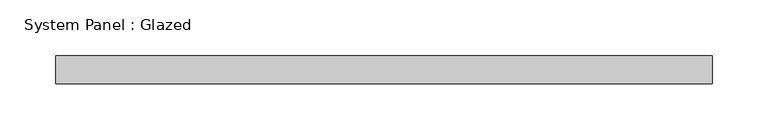
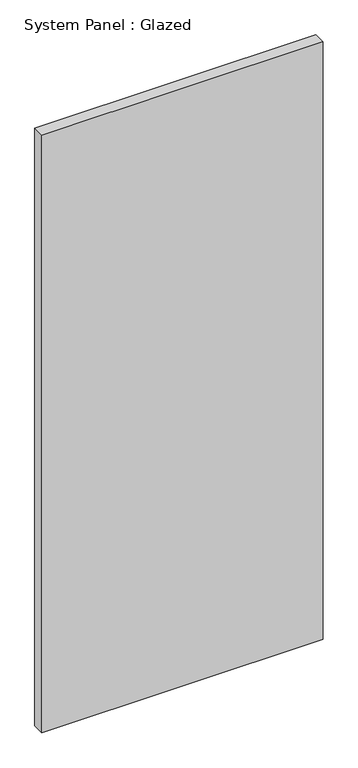
"""IFC4 building model written with IfcOpenShell, lengths in millimetres: plate geometry, System Panel : Glazed."""

from ifc_helpers import new_model, si_unit, origin, origin_with_axes, place, context, project, spatial, polyline, outline, extrude, source, transform, mapped, element, save


def system_panel_glazed_469e0694(model_context):
    return source(origin(), model_context, "Body", "SweptSolid", [
        extrude(outline(polyline([(295.275, 19.05), (-295.275, 19.05), (-295.275, 44.45), (295.275, 44.45), (295.275, 19.05)])), origin_with_axes(), (0.0, 0.0, 1.0), 1327.3964565),
    ])


if __name__ == "__main__":
    model = new_model("IFC4")
    model_context = context("Model", 3, world=origin())
    ifc_project = project(units=[si_unit("LENGTHUNIT", "METRE", prefix="MILLI")], contexts=[model_context])
    site = spatial("IfcSite", under=ifc_project)
    building = spatial("IfcBuilding", under=site)
    placement = place(None, origin())
    system_panel_glazed_shape = system_panel_glazed_469e0694(model_context)
    element("IfcPlate", 1, ObjectType="System Panel : Glazed", at=placement, inside=building, context=model_context, shape_type="MappedRepresentation", body=[
        mapped(system_panel_glazed_shape, transform((0.0, 0.0, 0.0), x_axis=(1.0, 0.0, 0.0), y_axis=(0.0, 1.0, 0.0), z_axis=(0.0, 0.0, 1.0))),
    ])
    save(model, "model.ifc")

# Revit data of these elements
# Type "System Panel : Glazed"
#   Construction Type Id = "GSP4R"
#   Analytic Construction = "1/8 in Pilkington single glazing"
#   Visual Light Transmittance = 0.9
#   Solar Heat Gain Coefficient = 0.86
#   Heat Transfer Coefficient (U) = 1.18115 BTU/(h·ft²·°F)
#   Define Thermal Properties by = 1
# Element 1 (IfcPlate, "System Panel : Glazed")
#   Materials on its faces: "Glass"
# Materials
#   "Glass": class "Glass", colour RGB 0 128 192, transparency 0.75, Description = "Soda Lime Glass", Cost = 0
